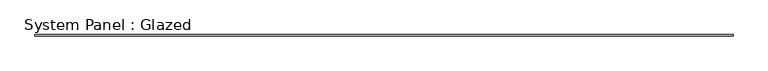
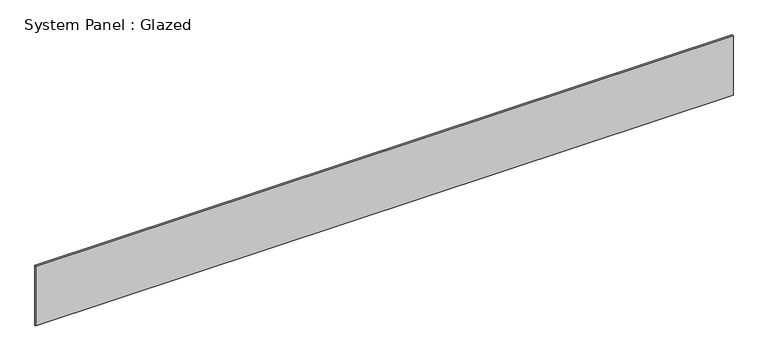
"""IFC4 building model written with IfcOpenShell, lengths in millimetres: plate geometry, System Panel : Glazed."""

from ifc_helpers import new_model, si_unit, origin, origin_with_axes, place, context, project, spatial, polyline, outline, extrude, source, transform, mapped, element, save


def system_panel_glazed_078a25c0(model_context):
    return source(origin(), model_context, "Body", "SweptSolid", [
        extrude(outline(polyline([(6378.8141536, 19.05), (-6378.8141536, 19.05), (-6378.8141536, 44.45), (6378.8141536, 44.45), (6378.8141536, 19.05)])), origin_with_axes(), (0.0, 0.0, 1.0), 1155.7),
    ])


if __name__ == "__main__":
    model = new_model("IFC4")
    model_context = context("Model", 3, world=origin())
    ifc_project = project(units=[si_unit("LENGTHUNIT", "METRE", prefix="MILLI")], contexts=[model_context])
    site = spatial("IfcSite", under=ifc_project)
    building = spatial("IfcBuilding", under=site)
    placement = place(None, origin())
    system_panel_glazed_shape = system_panel_glazed_078a25c0(model_context)
    element("IfcPlate", 1, ObjectType="System Panel : Glazed", at=placement, inside=building, context=model_context, shape_type="MappedRepresentation", body=[
        mapped(system_panel_glazed_shape, transform((0.0, 0.0, 0.0), x_axis=(1.0, 0.0, 0.0), y_axis=(0.0, 1.0, 0.0), z_axis=(0.0, 0.0, 1.0))),
    ])
    save(model, "model.ifc")

# Revit data of these elements
# Type "System Panel : Glazed"
#   Construction Type Id = "GSP4R"
#   Analytic Construction = "1/8 in Pilkington single glazing"
#   Visual Light Transmittance = 0.9
#   Solar Heat Gain Coefficient = 0.86
#   Heat Transfer Coefficient (U) = 1.18115 BTU/(h·ft²·°F)
# Element 1 (IfcPlate, "System Panel : Glazed")
#   Materials on its faces: "Glass"
# Materials
#   "Glass": class "Glass", colour RGB 0 128 192, transparency 0.75, Description = "Soda Lime Glass", Cost = 0
